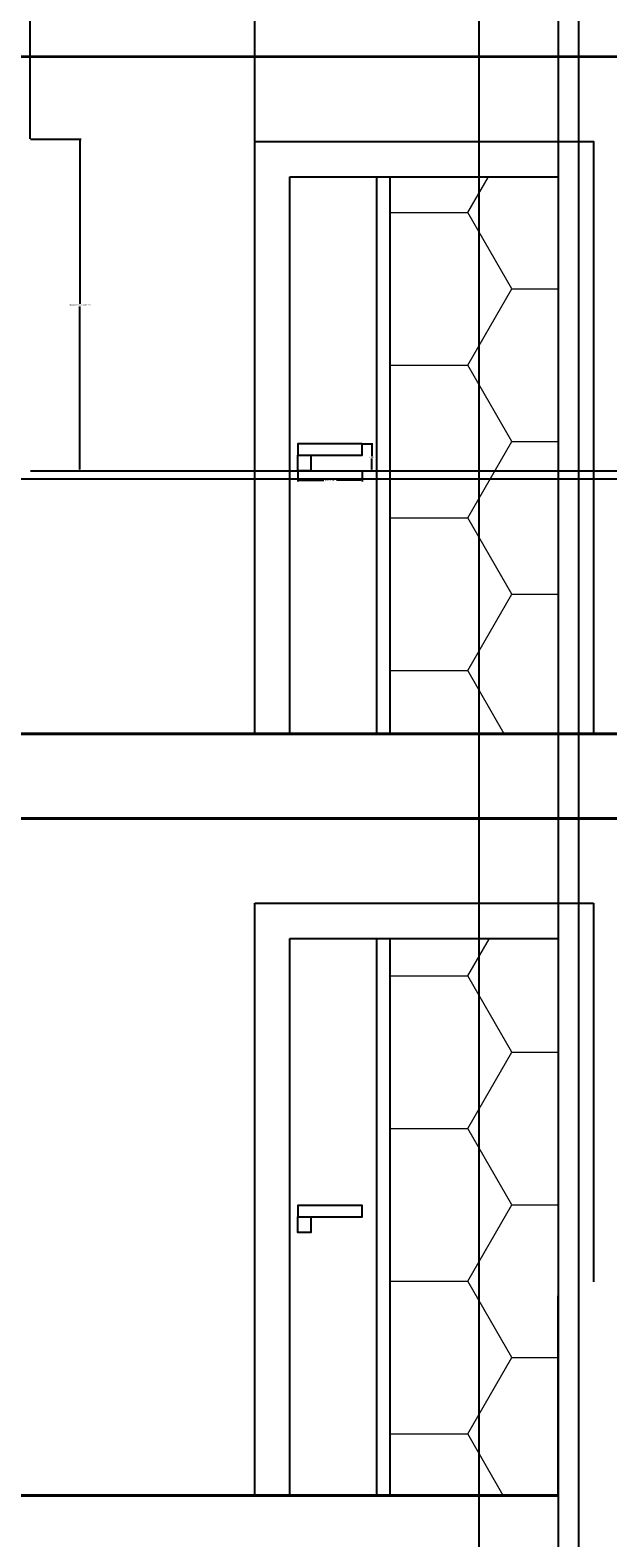
# Model space of a CAD drawing. Units: inches. Extents: x -8 to 554, y -200 to 499.
# Tile 10 of 12: x 358 to 440, y 121 to 335. Entities that reach past the tile are written whole.
import ezdxf

# ---------------------------------------------------------------- set-up
doc = ezdxf.new("R2010")
doc.units = ezdxf.units.IN
doc.header["$MEASUREMENT"] = 0
for name, color, linetype, lineweight in [('A-ANNO-DIMS', 2, 'Continuous', 18), ('A-DOOR', 3, 'Continuous', 25), ('A-DOOR-PATT', 252, 'Continuous', 13), ('A-FLOR', 7, 'Continuous', 35), ('A-WALL-PRPT', 7, 'Continuous', 25)]:
    doc.layers.add(name, color=color, linetype=linetype, lineweight=lineweight)
doc.styles.get("Standard").update_dxf_attribs({"font": 'arial.ttf'})
doc.dimstyles.get("Standard").update_dxf_attribs({"dimtxt": 0.18, "dimasz": 0.18, "dimexe": 0.18, "dimexo": 0.0625, "dimgap": 0.09, "dimtad": 0, "dimtih": 1, "dimtoh": 1, "dimdec": 4, "dimzin": 0, "dimdsep": 46, "dimtxsty": 'Standard', "dimcen": 0.09, "dimadec": 0, "dimazin": 0, "dimtfac": 1, "dimtdec": 4, "dimtofl": 0, "dimtmove": 0, "dimatfit": 3, "dimfxl": 1, "dimtolj": 1, "dimtzin": 0, "dimarcsym": 0})

# ---------------------------------------------------------------- blocks, each defined once
blk = doc.blocks.new('DOOR-LEVER-ELEV')
for points in [[(0, 2.19), (9.08, 2.19), (9.08, 3.81), (0, 3.81)], [(0, 2.19), (1.8, 2.19), (1.8, 0), (0, 0)]]:
    blk.add_lwpolyline(points, close=True)
blk = doc.blocks.new('*D16')
at = {"layer": 'A-ANNO-DIMS', "color": 0, "lineweight": -2, "transparency": 16777216}
for p, q in [((395.65, 272.73), (395.65, 271.25)), ((404.73, 272.73), (404.73, 271.25)), ((395.83, 271.43), (399.29, 271.43)), ((404.55, 271.43), (401.09, 271.43))]:
    blk.add_line(p, q, dxfattribs=at)
at = {"layer": 'A-ANNO-DIMS', "color": 0, "transparency": 16777216}
for points in [[(395.83, 271.46), (395.83, 271.4), (395.65, 271.43)], [(404.55, 271.46), (404.55, 271.4), (404.73, 271.43)]]:
    blk.add_solid(points, dxfattribs=at)
at = {"layer": 'Defpoints', "color": 0, "transparency": 16777216}
for p in [(395.65, 272.79), (404.73, 272.79), (404.73, 271.43)]:
    blk.add_point(p, dxfattribs=at)
at = {"layer": 'A-ANNO-DIMS', "color": 0, "transparency": 16777216, "insert": (400.19, 271.43), "char_height": 0.18, "attachment_point": 5}
blk.add_mtext('\\A1;LEVER 9 TYP.', dxfattribs=at)
blk = doc.blocks.new('*D17')
at = {"layer": 'A-ANNO-DIMS', "color": 0, "lineweight": -2, "transparency": 16777216}
for p, q in [((404.8, 276.6), (406.28, 276.6)), ((406.1, 276.42), (406.1, 274.87)), ((406.1, 272.97), (406.1, 274.51)), ((404.8, 272.79), (406.28, 272.79))]:
    blk.add_line(p, q, dxfattribs=at)
at = {"layer": 'A-ANNO-DIMS', "color": 0, "transparency": 16777216}
for points in [[(406.07, 276.42), (406.13, 276.42), (406.1, 276.6)], [(406.07, 272.97), (406.13, 272.97), (406.1, 272.79)]]:
    blk.add_solid(points, dxfattribs=at)
at = {"layer": 'Defpoints', "color": 0, "transparency": 16777216}
for p in [(404.73, 276.6), (406.1, 276.6), (404.73, 272.79)]:
    blk.add_point(p, dxfattribs=at)
at = {"layer": 'A-ANNO-DIMS', "color": 0, "transparency": 16777216, "insert": (406.1, 274.69), "char_height": 0.18, "attachment_point": 5}
blk.add_mtext('\\A1;4 TYP.', dxfattribs=at)
blk = doc.blocks.new('*D26')
at = {"layer": 'A-ANNO-DIMS', "color": 0, "lineweight": -2, "transparency": 16777216}
for p, q in [((357.76, 319.79), (364.93, 319.79)), ((364.75, 319.61), (364.75, 296.46)), ((364.75, 272.94), (364.75, 296.09)), ((357.76, 272.76), (364.93, 272.76))]:
    blk.add_line(p, q, dxfattribs=at)
at = {"layer": 'A-ANNO-DIMS', "color": 0, "transparency": 16777216}
for points in [[(364.72, 319.61), (364.78, 319.61), (364.75, 319.79)], [(364.72, 272.94), (364.78, 272.94), (364.75, 272.76)]]:
    blk.add_solid(points, dxfattribs=at)
at = {"layer": 'Defpoints', "color": 0, "transparency": 16777216}
for p in [(357.7, 319.79), (364.75, 319.79), (357.7, 272.76)]:
    blk.add_point(p, dxfattribs=at)
at = {"layer": 'A-ANNO-DIMS', "color": 0, "transparency": 16777216, "insert": (364.75, 296.28), "char_height": 0.18, "attachment_point": 5}
blk.add_mtext('\\A1;TWO-LIGHT CASING 47 TYP.', dxfattribs=at)
blk = doc.blocks.new('*D31')
at = {"layer": 'A-ANNO-DIMS', "color": 0, "lineweight": -2, "transparency": 16777216}
for p, q in [((24.34, 127.42), (24.34, -199.97)), ((453.32, -30.73), (453.32, -199.97)), ((24.52, -199.79), (238.54, -199.79)), ((453.14, -199.79), (239.12, -199.79))]:
    blk.add_line(p, q, dxfattribs=at)
at = {"layer": 'A-ANNO-DIMS', "color": 0, "transparency": 16777216}
for points in [[(24.52, -199.76), (24.52, -199.82), (24.34, -199.79)], [(453.14, -199.76), (453.14, -199.82), (453.32, -199.79)]]:
    blk.add_solid(points, dxfattribs=at)
at = {"layer": 'Defpoints', "color": 0, "transparency": 16777216}
for p in [(24.34, 127.48), (453.32, -30.67), (453.32, -199.79)]:
    blk.add_point(p, dxfattribs=at)
at = {"layer": 'A-ANNO-DIMS', "color": 0, "transparency": 16777216, "insert": (238.83, -199.79), "char_height": 0.18, "attachment_point": 5}
blk.add_mtext('\\A1;429', dxfattribs=at)
blk = doc.blocks.new('*D32')
at = {"layer": 'A-ANNO-DIMS', "color": 0, "lineweight": -2, "transparency": 16777216}
for p, q in [((24.34, 223.42), (24.34, -199.97)), ((444.34, 223.42), (444.34, -199.97)), ((24.52, -199.79), (234.05, -199.79)), ((444.16, -199.79), (234.63, -199.79))]:
    blk.add_line(p, q, dxfattribs=at)
at = {"layer": 'A-ANNO-DIMS', "color": 0, "transparency": 16777216}
for points in [[(24.52, -199.76), (24.52, -199.82), (24.34, -199.79)], [(444.16, -199.76), (444.16, -199.82), (444.34, -199.79)]]:
    blk.add_solid(points, dxfattribs=at)
at = {"layer": 'Defpoints', "color": 0, "transparency": 16777216}
for p in [(24.34, 223.48), (444.34, 223.48), (444.34, -199.79)]:
    blk.add_point(p, dxfattribs=at)
at = {"layer": 'A-ANNO-DIMS', "color": 0, "transparency": 16777216, "insert": (234.34, -199.79), "char_height": 0.18, "attachment_point": 5}
blk.add_mtext('\\A1;420', dxfattribs=at)
blk = doc.blocks.new('*D45')
at = {"layer": 'A-ANNO-DIMS', "color": 0, "lineweight": -2, "transparency": 16777216}
for p, q in [((357.7, 319.85), (357.7, 498.99)), ((357.88, 498.81), (373.22, 498.81)), ((389.34, 498.81), (374, 498.81)), ((389.52, 319.54), (389.52, 498.99))]:
    blk.add_line(p, q, dxfattribs=at)
at = {"layer": 'A-ANNO-DIMS', "color": 0, "transparency": 16777216}
for points in [[(357.88, 498.84), (357.88, 498.78), (357.7, 498.81)], [(389.34, 498.84), (389.34, 498.78), (389.52, 498.81)]]:
    blk.add_solid(points, dxfattribs=at)
at = {"layer": 'Defpoints', "color": 0, "transparency": 16777216}
for p in [(389.52, 498.81), (357.7, 319.79), (389.52, 319.48)]:
    blk.add_point(p, dxfattribs=at)
at = {"layer": 'A-ANNO-DIMS', "color": 0, "transparency": 16777216, "insert": (373.61, 498.81), "char_height": 0.18, "attachment_point": 5}
blk.add_mtext('\\A1;31.82', dxfattribs=at)
blk = doc.blocks.new('*D46')
at = {"layer": 'A-ANNO-DIMS', "color": 0, "lineweight": -2, "transparency": 16777216}
for p, q in [((101.04, 271.66), (554.26, 271.66)), ((554.08, 271.48), (554.08, 253.75)), ((554.08, 235.66), (554.08, 253.39)), ((66.27, 235.48), (554.26, 235.48))]:
    blk.add_line(p, q, dxfattribs=at)
at = {"layer": 'A-ANNO-DIMS', "color": 0, "transparency": 16777216}
for points in [[(554.05, 271.48), (554.11, 271.48), (554.08, 271.66)], [(554.05, 235.66), (554.11, 235.66), (554.08, 235.48)]]:
    blk.add_solid(points, dxfattribs=at)
at = {"layer": 'Defpoints', "color": 0, "transparency": 16777216}
for p in [(100.98, 271.66), (66.2, 235.48), (554.08, 235.48)]:
    blk.add_point(p, dxfattribs=at)
at = {"layer": 'A-ANNO-DIMS', "color": 0, "transparency": 16777216, "insert": (554.08, 253.57), "char_height": 0.18, "attachment_point": 5}
blk.add_mtext('\\A1;36.18', dxfattribs=at)
blk = doc.blocks.new('*D47')
at = {"layer": 'A-ANNO-DIMS', "color": 0, "lineweight": -2, "transparency": 16777216}
for p, q in [((357.76, 272.76), (554.26, 272.76)), ((554.08, 272.58), (554.08, 254.3)), ((554.08, 235.66), (554.08, 253.94)), ((312.4, 235.48), (554.26, 235.48))]:
    blk.add_line(p, q, dxfattribs=at)
at = {"layer": 'A-ANNO-DIMS', "color": 0, "transparency": 16777216}
for points in [[(554.05, 272.58), (554.11, 272.58), (554.08, 272.76)], [(554.05, 235.66), (554.11, 235.66), (554.08, 235.48)]]:
    blk.add_solid(points, dxfattribs=at)
at = {"layer": 'Defpoints', "color": 0, "transparency": 16777216}
for p in [(357.7, 272.76), (312.34, 235.48), (554.08, 235.48)]:
    blk.add_point(p, dxfattribs=at)
at = {"layer": 'A-ANNO-DIMS', "color": 0, "transparency": 16777216, "insert": (554.08, 254.12), "char_height": 0.18, "attachment_point": 5}
blk.add_mtext('\\A1;37.28', dxfattribs=at)
blk = doc.blocks.new('*D55')
at = {"layer": 'A-ANNO-DIMS', "color": 0, "lineweight": -2, "transparency": 16777216}
for p, q in [((204.61, -30.61), (204.61, 498.99)), ((204.79, 498.81), (328.57, 498.81)), ((453.14, 498.81), (329.36, 498.81)), ((453.32, -30.61), (453.32, 498.99))]:
    blk.add_line(p, q, dxfattribs=at)
at = {"layer": 'A-ANNO-DIMS', "color": 0, "transparency": 16777216}
for points in [[(204.79, 498.84), (204.79, 498.78), (204.61, 498.81)], [(453.14, 498.84), (453.14, 498.78), (453.32, 498.81)]]:
    blk.add_solid(points, dxfattribs=at)
at = {"layer": 'Defpoints', "color": 0, "transparency": 16777216}
for p in [(453.32, 498.81), (204.61, -30.67), (453.32, -30.67)]:
    blk.add_point(p, dxfattribs=at)
at = {"layer": 'A-ANNO-DIMS', "color": 0, "transparency": 16777216, "insert": (328.96, 498.81), "char_height": 0.18, "attachment_point": 5}
blk.add_mtext('\\A1;248.7', dxfattribs=at)
blk = doc.blocks.new('*D64')
at = {"layer": 'A-ANNO-DIMS', "color": 0, "lineweight": -2, "transparency": 16777216}
for p, q in [((337.49, 7.54), (337.49, 498.99)), ((337.67, 498.81), (379.02, 498.81)), ((421.13, 498.81), (379.78, 498.81)), ((421.31, 7.54), (421.31, 498.99))]:
    blk.add_line(p, q, dxfattribs=at)
at = {"layer": 'A-ANNO-DIMS', "color": 0, "transparency": 16777216}
for points in [[(337.67, 498.84), (337.67, 498.78), (337.49, 498.81)], [(421.13, 498.84), (421.13, 498.78), (421.31, 498.81)]]:
    blk.add_solid(points, dxfattribs=at)
at = {"layer": 'Defpoints', "color": 0, "transparency": 16777216}
for p in [(421.31, 498.81), (337.49, 7.48), (421.31, 7.48)]:
    blk.add_point(p, dxfattribs=at)
at = {"layer": 'A-ANNO-DIMS', "color": 0, "transparency": 16777216, "insert": (379.4, 498.81), "char_height": 0.18, "attachment_point": 5}
blk.add_mtext('\\A1;83.81', dxfattribs=at)
blk = doc.blocks.new('*D65')
at = {"layer": 'A-ANNO-DIMS', "color": 0, "lineweight": -2, "transparency": 16777216}
for p, q in [((421.31, 7.54), (421.31, 498.99)), ((421.49, 498.81), (428, 498.81)), ((435.29, 498.81), (428.77, 498.81)), ((435.47, 7.54), (435.47, 498.99))]:
    blk.add_line(p, q, dxfattribs=at)
at = {"layer": 'A-ANNO-DIMS', "color": 0, "transparency": 16777216}
for points in [[(421.49, 498.84), (421.49, 498.78), (421.31, 498.81)], [(435.29, 498.84), (435.29, 498.78), (435.47, 498.81)]]:
    blk.add_solid(points, dxfattribs=at)
at = {"layer": 'Defpoints', "color": 0, "transparency": 16777216}
for p in [(435.47, 498.81), (421.31, 7.48), (435.47, 7.48)]:
    blk.add_point(p, dxfattribs=at)
at = {"layer": 'A-ANNO-DIMS', "color": 0, "transparency": 16777216, "insert": (428.39, 498.81), "char_height": 0.18, "attachment_point": 5}
blk.add_mtext('\\A1;14.16', dxfattribs=at)
blk = doc.blocks.new('*D71')
at = {"layer": 'A-ANNO-DIMS', "color": 0, "lineweight": -2, "transparency": 16777216}
for p, q in [((444.34, 439.42), (444.34, -199.97)), ((432.52, 427.42), (432.52, -199.97)), ((432.7, -199.79), (437.97, -199.79)), ((444.16, -199.79), (438.89, -199.79))]:
    blk.add_line(p, q, dxfattribs=at)
at = {"layer": 'A-ANNO-DIMS', "color": 0, "transparency": 16777216}
for points in [[(432.7, -199.76), (432.7, -199.82), (432.52, -199.79)], [(444.16, -199.76), (444.16, -199.82), (444.34, -199.79)]]:
    blk.add_solid(points, dxfattribs=at)
at = {"layer": 'Defpoints', "color": 0, "transparency": 16777216}
for p in [(444.34, 439.48), (432.52, 427.48), (444.34, -199.79)]:
    blk.add_point(p, dxfattribs=at)
at = {"layer": 'A-ANNO-DIMS', "color": 0, "transparency": 16777216, "insert": (438.43, -199.79), "char_height": 0.18, "attachment_point": 5}
blk.add_mtext('\\A1;11.825', dxfattribs=at)

msp = doc.modelspace()

# ---------------------------------------------------------------- hatches: boundary and pattern name
at = {"layer": 'A-DOOR-PATT', "transparency": 33554523}
h = msp.add_hatch(dxfattribs=at)
h.set_pattern_fill('HONEY', color=256, scale=100)
h.set_pattern_definition([(0, (-117.809, -80.312), (18.75, 10.82532), [12.5, -25]), (120, (-117.809, -80.312), (-18.75, 10.82532), [12.5, -25]), (60, (-117.809, -80.312), (4e-15, 21.65064), [-25, 12.5])])
h.paths.add_polyline_path([(211.3421, 314.4814), (187.4809, 314.4814), (187.4809, 235.4814), (211.3421, 235.4814)])
h.paths.add_polyline_path([(211.3421, 206.4814), (187.4809, 206.4814), (187.4809, 127.4814), (211.3421, 127.4814)])
h.paths.add_polyline_path([(211.3421, 98.4814), (187.4809, 98.4814), (187.4809, 19.4814), (211.3421, 19.4814)])
h.paths.add_polyline_path([(432.5174, 98.4814), (408.6562, 98.4814), (408.6562, 19.4814), (432.5174, 19.4814)])
h.paths.add_polyline_path([(432.5174, 206.4814), (408.6562, 206.4814), (408.6562, 127.4814), (432.5174, 127.4814), (432.5174, 155.7921)])
h.paths.add_polyline_path([(432.5174, 314.4814), (408.6562, 314.4814), (408.6562, 235.4814), (432.5174, 235.4814)])

# ---------------------------------------------------------------- linework, layer by layer
at = {"layer": 'A-DOOR'}
for p, q in [((394.5174, 235.4814), (394.5174, 314.4814)), ((394.5174, 314.4814), (432.5174, 314.4814)), ((432.5174, 314.4814), (432.5174, 235.4814)), ((389.5174, 127.4814), (389.5174, 211.4814)), ((389.5174, 211.4814), (437.5174, 211.4814)), ((437.5174, 211.4814), (437.5174, 157.7921)), ((394.5174, 127.4814), (394.5174, 206.4814)), ((394.5174, 206.4814), (432.5174, 206.4814)), ((432.5174, 206.4814), (432.5174, 127.4814)), ((432.5174, 127.4814), (389.5174, 127.4814))]:
    msp.add_line(p, q, dxfattribs=at)
for points in [[(437.5174, 235.4814), (389.5174, 235.4814), (389.5174, 319.4814), (437.5174, 319.4814)], [(406.8193, 314.4814), (408.6562, 314.4814), (408.6562, 235.4814), (406.8193, 235.4814)], [(406.8193, 206.4814), (408.6562, 206.4814), (408.6562, 127.4814), (406.8193, 127.4814)]]:
    msp.add_lwpolyline(points, close=True, dxfattribs=at)
at = {"layer": 'A-FLOR'}
for p, q in [((444.3421, 331.4814), (36.3421, 331.4814)), ((444.3421, 235.4814), (24.3421, 235.4814)), ((36.3421, 235.4814), (444.3421, 235.4814)), ((24.3421, 223.4814), (444.3421, 223.4814)), ((444.3421, 223.4814), (36.3421, 223.4814)), ((432.5174, 127.4814), (24.3421, 127.4814)), ((36.3421, 127.4814), (432.5174, 127.4814))]:
    msp.add_line(p, q, dxfattribs=at)
at = {"layer": 'A-WALL-PRPT'}
msp.add_lwpolyline([(432.5174, 127.4814), (432.5174, 155.7921)], dxfattribs=at)

# ---------------------------------------------------------------- block references
at = {"layer": 'A-DOOR'}
for p in [(395.6515, 272.7884), (395.6515, 164.7884)]:
    msp.add_blockref('DOOR-LEVER-ELEV', p, dxfattribs=at)

# ---------------------------------------------------------------- dimensions: what is measured, and where the dimension line sits
at = {"layer": 'A-ANNO-DIMS'}
for base, p1, p2, override, picture, middle in [((453.3222, 498.8091), (204.6055, -30.6677), (453.3222, -30.6677), {"dimdec": 1, "dimlfac": 1, "dimrnd": 0, "dimzin": 0, "dimdsep": 46, "dimlunit": 2}, '*D55', (328.9639, 498.8091)), ((421.3053, 498.8091), (337.4923, 7.4814), (421.3053, 7.4814), {"dimdec": 2, "dimlfac": 1, "dimrnd": 0, "dimzin": 0, "dimdsep": 46, "dimlunit": 2}, '*D64', (379.3988, 498.8091)), ((389.5174, 498.8091), (357.699, 319.788), (389.5174, 319.4814), {"dimdec": 2, "dimlfac": 1, "dimrnd": 0, "dimzin": 0, "dimdsep": 46, "dimlunit": 2}, '*D45', (373.6082, 498.8091)), ((435.4655, 498.8091), (421.3053, 7.4814), (435.4655, 7.4814), {"dimdec": 2, "dimlfac": 1, "dimrnd": 0, "dimzin": 0, "dimdsep": 46, "dimlunit": 2}, '*D65', (428.3854, 498.8091)), ((444.3421, -199.7912), (432.5174, 427.4814), (444.3421, 439.4814), {"dimdec": 3, "dimlfac": 1, "dimrnd": 0, "dimzin": 0, "dimdsep": 46, "dimlunit": 2}, '*D71', (438.4297, -199.7912)), ((444.3421, -199.7912), (24.3421, 223.4814), (444.3421, 223.4814), {"dimdec": 0, "dimlfac": 1, "dimrnd": 0, "dimzin": 0, "dimdsep": 46, "dimlunit": 2}, '*D32', (234.3421, -199.7912)), ((453.3222, -199.7912), (24.3421, 127.4814), (453.3222, -30.6677), {"dimdec": 0, "dimlfac": 1, "dimrnd": 0, "dimzin": 0, "dimdsep": 46, "dimlunit": 2}, '*D31', (238.8321, -199.7912))]:
    dim = msp.add_linear_dim(base=base, p1=p1, p2=p2, dimstyle='Standard', override=override, dxfattribs=at)
    dim.commit()
    dim.dimension.update_dxf_attribs({"geometry": picture, "text_midpoint": middle})
for base, p1, p2, text, picture, middle in [((364.7529, 319.788), (357.699, 272.7623), (357.699, 319.788), 'TWO-LIGHT CASING <> TYP.', '*D26', (364.7529, 296.2752)), ((406.0967, 276.5985), (404.7343, 272.7884), (404.7343, 276.5985), '<> TYP.', '*D17', (406.0967, 274.6935))]:
    dim = msp.add_linear_dim(base=base, p1=p1, p2=p2, angle=90, text=text, dimstyle='Standard', override={"dimdec": 0, "dimlfac": 1, "dimrnd": 0, "dimzin": 0, "dimdsep": 46, "dimlunit": 2}, dxfattribs=at)
    dim.commit()
    dim.dimension.update_dxf_attribs({"geometry": picture, "text_midpoint": middle})
for p1, p2, picture, middle in [((100.9765, 271.661), (66.2048, 235.4814), '*D46', (554.0833, 253.5712)), ((357.699, 272.7623), (312.3421, 235.4814), '*D47', (554.0833, 254.1218))]:
    dim = msp.add_linear_dim(base=(554.0833, 235.4814), p1=p1, p2=p2, angle=90, dimstyle='Standard', override={"dimdec": 2, "dimlfac": 1, "dimrnd": 0, "dimzin": 0, "dimdsep": 46, "dimlunit": 2}, dxfattribs=at)
    dim.commit()
    dim.dimension.update_dxf_attribs({"geometry": picture, "text_midpoint": middle})
dim = msp.add_linear_dim(base=(404.7343, 271.426), p1=(395.6515, 272.7884), p2=(404.7343, 272.7884), text='LEVER <> TYP.', dimstyle='Standard', override={"dimdec": 0, "dimlfac": 1, "dimrnd": 0, "dimzin": 0, "dimdsep": 46, "dimlunit": 2}, dxfattribs=at)
dim.commit()
dim.dimension.update_dxf_attribs({"geometry": '*D16', "text_midpoint": (400.1929, 271.426)})

doc.saveas('drawing.dxf')
